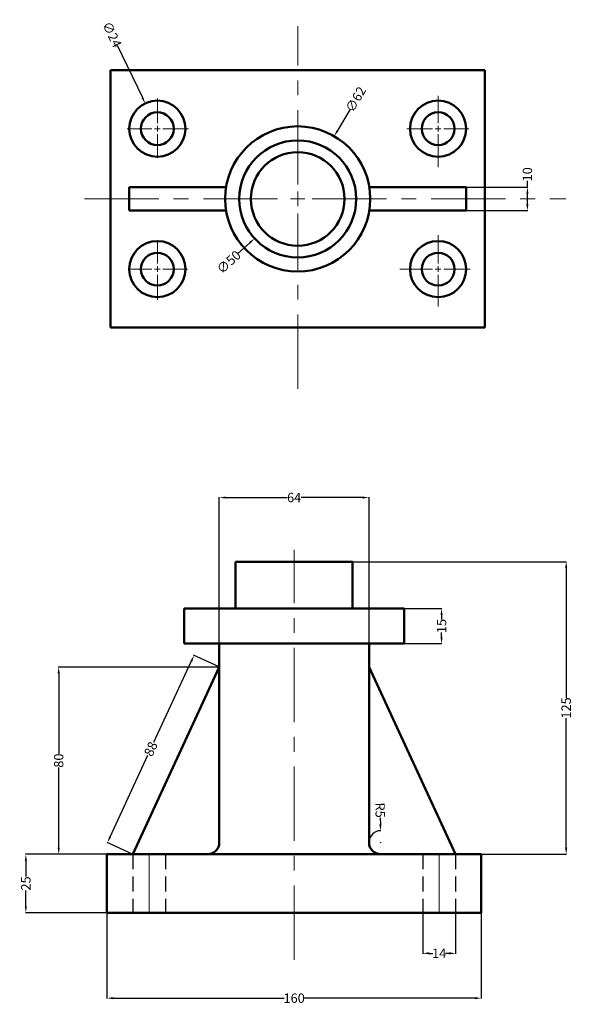
# Model space of a CAD drawing. Units: inches. Extents: x 680 to 916, y 368 to 789.
import ezdxf

# ---------------------------------------------------------------- set-up
doc = ezdxf.new("R2010")
doc.units = ezdxf.units.IN
doc.header["$MEASUREMENT"] = 0
doc.linetypes.add('CENTER', pattern=[50.8, 31.75, -6.35, 6.35, -6.35])
doc.linetypes.add('HIDDEN', pattern=[9.525, 6.35, -3.175])
for name, color, linetype, lineweight in [('M-CNTR', 1, 'CENTER', 18), ('M-DIMS', 2, 'Continuous', 25), ('M-HIDN', 6, 'HIDDEN', 25), ('M-OUTL', 7, 'Continuous', 50)]:
    doc.layers.add(name, color=color, linetype=linetype, lineweight=lineweight)
doc.styles.get("Standard").update_dxf_attribs({"font": 'arial.ttf'})
doc.dimstyles.get("Standard").update_dxf_attribs({"dimtxt": 4, "dimasz": 2.75, "dimexe": 0.18, "dimexo": 0.0625, "dimgap": 0.09, "dimtad": 0, "dimdec": 0, "dimzin": 0, "dimdsep": 46, "dimtxsty": 'Standard', "dimcen": 0.09, "dimadec": 0, "dimazin": 0, "dimtfac": 1, "dimtdec": 0, "dimtofl": 0, "dimtmove": 0, "dimatfit": 3, "dimfxl": 1, "dimtolj": 1, "dimtzin": 0, "dimarcsym": 0})

# ---------------------------------------------------------------- blocks, each defined once
blk = doc.blocks.new('*U1')
at = {"layer": 'M-CNTR', "color": 0, "transparency": 16777216}
for p, q in [((0, 2.4), (0, 12.94)), ((-12.91, 0), (-2.4, 0)), ((2.4, 0), (13.36, 0)), ((0, -12.46), (0, -2.4))]:
    blk.add_line(p, q, dxfattribs=at)
at = {"layer": 'M-CNTR', "color": 0, "linetype": 'Continuous', "transparency": 16777216}
for p, q in [((-1.2, 0), (1.2, 0)), ((0, -1.2), (0, 1.2))]:
    blk.add_line(p, q, dxfattribs=at)
blk = doc.blocks.new('*U2')
at = {"layer": 'M-CNTR', "color": 0, "transparency": 16777216}
for p, q in [((0, 2.4), (0, 12.35)), ((-12.5, 0), (-2.4, 0)), ((2.4, 0), (12.96, 0)), ((0, -13.15), (0, -2.4))]:
    blk.add_line(p, q, dxfattribs=at)
at = {"layer": 'M-CNTR', "color": 0, "linetype": 'Continuous', "transparency": 16777216}
for p, q in [((-1.2, 0), (1.2, 0)), ((0, -1.2), (0, 1.2))]:
    blk.add_line(p, q, dxfattribs=at)
blk = doc.blocks.new('*U3')
at = {"layer": 'M-CNTR', "color": 0, "transparency": 16777216}
for p, q in [((0, 2.4), (0, 14.5)), ((-16.29, 0), (-2.4, 0)), ((2.4, 0), (13.65, 0)), ((0, -15.95), (0, -2.4))]:
    blk.add_line(p, q, dxfattribs=at)
at = {"layer": 'M-CNTR', "color": 0, "linetype": 'Continuous', "transparency": 16777216}
for p, q in [((-1.2, 0), (1.2, 0)), ((0, -1.2), (0, 1.2))]:
    blk.add_line(p, q, dxfattribs=at)
blk = doc.blocks.new('*U4')
at = {"layer": 'M-CNTR', "color": 0, "transparency": 16777216}
for p, q in [((0, 2.4), (0, 13.99)), ((-13.32, 0), (-2.4, 0)), ((2.4, 0), (13.15, 0)), ((0, -16.48), (0, -2.4))]:
    blk.add_line(p, q, dxfattribs=at)
at = {"layer": 'M-CNTR', "color": 0, "linetype": 'Continuous', "transparency": 16777216}
for p, q in [((-1.2, 0), (1.2, 0)), ((0, -1.2), (0, 1.2))]:
    blk.add_line(p, q, dxfattribs=at)
blk = doc.blocks.new('*U5')
at = {"layer": 'M-CNTR', "color": 0, "transparency": 16777216}
for p, q in [((0, 6.2), (0, 73.87)), ((-91.14, 0), (-6.2, 0)), ((6.2, 0), (114.65, 0)), ((0, -81.14), (0, -6.2))]:
    blk.add_line(p, q, dxfattribs=at)
at = {"layer": 'M-CNTR', "color": 0, "linetype": 'Continuous', "transparency": 16777216}
for p, q in [((-3.1, 0), (3.1, 0)), ((0, -3.1), (0, 3.1))]:
    blk.add_line(p, q, dxfattribs=at)
blk = doc.blocks.new('*D6')
at = {"layer": 'Defpoints', "color": 0, "transparency": 16777216}
for p in [(871.07, 717.23), (897.24, 717.23), (871.07, 707.23)]:
    blk.add_point(p, dxfattribs=at)
at = {"layer": 'M-DIMS', "color": 0, "lineweight": -2, "transparency": 16777216}
for p, q in [((897.24, 717.23), (897.24, 719.98)), ((871.13, 717.23), (897.42, 717.23)), ((897.24, 709.98), (897.24, 714.48)), ((871.13, 707.23), (897.42, 707.23))]:
    blk.add_line(p, q, dxfattribs=at)
at = {"layer": 'M-DIMS', "color": 0, "transparency": 16777216}
for points in [[(896.78, 714.48), (897.7, 714.48), (897.24, 717.23)], [(896.78, 709.98), (897.7, 709.98), (897.24, 707.23)]]:
    blk.add_solid(points, dxfattribs=at)
at = {"layer": 'M-DIMS', "color": 0, "transparency": 16777216, "insert": (897.24, 722.74), "char_height": 4, "attachment_point": 5, "rotation": 90}
blk.add_mtext('\\A1;10', dxfattribs=at)
blk = doc.blocks.new('*D7')
at = {"layer": 'Defpoints', "color": 0, "transparency": 16777216}
for p in [(814.69, 739.04), (783.44, 685.43)]:
    blk.add_point(p, dxfattribs=at)
at = {"layer": 'M-DIMS', "color": 0, "lineweight": -2, "transparency": 16777216}
for p, q in [((821.28, 750.35), (816.07, 741.41)), ((798.98, 712.23), (799.16, 712.23)), ((799.07, 712.14), (799.07, 712.32))]:
    blk.add_line(p, q, dxfattribs=at)
at = {"layer": 'M-DIMS', "color": 0, "transparency": 16777216}
blk.add_solid([(815.68, 741.64), (816.47, 741.18), (814.69, 739.04)], dxfattribs=at)
at = {"layer": 'M-DIMS', "color": 0, "transparency": 16777216, "insert": (823.85, 754.76), "char_height": 4, "attachment_point": 5, "rotation": 59.7637}
blk.add_mtext('\\A1;∅62', dxfattribs=at)
blk = doc.blocks.new('*D8')
at = {"layer": 'Defpoints', "color": 0, "transparency": 16777216}
for p in [(817.5, 729.12), (780.63, 695.35)]:
    blk.add_point(p, dxfattribs=at)
at = {"layer": 'M-DIMS', "color": 0, "lineweight": -2, "transparency": 16777216}
for p, q in [((798.98, 712.23), (799.16, 712.23)), ((799.07, 712.14), (799.07, 712.32)), ((773.36, 688.7), (778.6, 693.49))]:
    blk.add_line(p, q, dxfattribs=at)
at = {"layer": 'M-DIMS', "color": 0, "transparency": 16777216}
blk.add_solid([(778.29, 693.83), (778.91, 693.15), (780.63, 695.35)], dxfattribs=at)
at = {"layer": 'M-DIMS', "color": 0, "transparency": 16777216, "insert": (769.58, 685.24), "char_height": 4, "attachment_point": 5, "rotation": 42.4796}
blk.add_mtext('\\A1;∅50', dxfattribs=at)
blk = doc.blocks.new('*D9')
at = {"layer": 'Defpoints', "color": 0, "transparency": 16777216}
for p in [(733.86, 753.05), (744.27, 731.42)]:
    blk.add_point(p, dxfattribs=at)
at = {"layer": 'M-DIMS', "color": 0, "lineweight": -2, "transparency": 16777216}
for p, q in [((721.91, 777.88), (732.67, 755.52)), ((738.98, 742.23), (739.16, 742.23)), ((739.07, 742.14), (739.07, 742.32))]:
    blk.add_line(p, q, dxfattribs=at)
at = {"layer": 'M-DIMS', "color": 0, "transparency": 16777216}
blk.add_solid([(733.08, 755.72), (732.26, 755.33), (733.86, 753.05)], dxfattribs=at)
at = {"layer": 'M-DIMS', "color": 0, "transparency": 16777216, "insert": (719.69, 782.49), "char_height": 4, "attachment_point": 5, "rotation": 295.7004}
blk.add_mtext('\\A1;∅24', dxfattribs=at)
blk = doc.blocks.new('*U10')
at = {"layer": 'M-CNTR', "color": 0, "transparency": 16777216}
blk.add_line((0, -87.62), (0, 87.62), dxfattribs=at)
blk = doc.blocks.new('*D11')
at = {"layer": 'Defpoints', "color": 0, "transparency": 16777216}
for p in [(829.54, 584.6), (765.54, 522.18), (829.54, 522.18)]:
    blk.add_point(p, dxfattribs=at)
at = {"layer": 'M-DIMS', "color": 0, "lineweight": -2, "transparency": 16777216}
for p, q in [((765.54, 522.24), (765.54, 584.78)), ((768.29, 584.6), (794.58, 584.6)), ((826.79, 584.6), (800.5, 584.6)), ((829.54, 522.24), (829.54, 584.78))]:
    blk.add_line(p, q, dxfattribs=at)
at = {"layer": 'M-DIMS', "color": 0, "transparency": 16777216}
for points in [[(768.29, 585.06), (768.29, 584.15), (765.54, 584.6)], [(826.79, 585.06), (826.79, 584.15), (829.54, 584.6)]]:
    blk.add_solid(points, dxfattribs=at)
at = {"layer": 'M-DIMS', "color": 0, "transparency": 16777216, "insert": (797.54, 584.6), "char_height": 4, "attachment_point": 5}
blk.add_mtext('\\A1;64', dxfattribs=at)
blk = doc.blocks.new('*D12')
at = {"layer": 'Defpoints', "color": 0, "transparency": 16777216}
for p in [(765.54, 512.18), (696.9, 432.18), (765.54, 432.18)]:
    blk.add_point(p, dxfattribs=at)
at = {"layer": 'M-DIMS', "color": 0, "lineweight": -2, "transparency": 16777216}
for p, q in [((765.48, 512.18), (696.72, 512.18)), ((696.9, 509.43), (696.9, 475.13)), ((696.9, 434.93), (696.9, 469.23)), ((765.48, 432.18), (696.72, 432.18))]:
    blk.add_line(p, q, dxfattribs=at)
at = {"layer": 'M-DIMS', "color": 0, "transparency": 16777216}
for points in [[(696.44, 509.43), (697.36, 509.43), (696.9, 512.18)], [(696.44, 434.93), (697.36, 434.93), (696.9, 432.18)]]:
    blk.add_solid(points, dxfattribs=at)
at = {"layer": 'M-DIMS', "color": 0, "transparency": 16777216, "insert": (696.9, 472.18), "char_height": 4, "attachment_point": 5, "rotation": 90}
blk.add_mtext('\\A1;80', dxfattribs=at)
blk = doc.blocks.new('*D13')
at = {"layer": 'Defpoints', "color": 0, "transparency": 16777216}
for p in [(765.54, 512.18), (717.75, 437.17), (728.54, 432.18)]:
    blk.add_point(p, dxfattribs=at)
at = {"layer": 'M-DIMS', "color": 0, "lineweight": -2, "transparency": 16777216}
for p, q in [((753.59, 514.67), (737.49, 479.85)), ((765.48, 512.2), (754.59, 517.24)), ((718.9, 439.66), (735.01, 474.48)), ((728.48, 432.2), (717.59, 437.24))]:
    blk.add_line(p, q, dxfattribs=at)
at = {"layer": 'M-DIMS', "color": 0, "transparency": 16777216}
for points in [[(753.18, 514.86), (754.01, 514.48), (754.75, 517.17)], [(718.49, 439.85), (719.32, 439.47), (717.75, 437.17)]]:
    blk.add_solid(points, dxfattribs=at)
at = {"layer": 'M-DIMS', "color": 0, "transparency": 16777216, "insert": (736.25, 477.17), "char_height": 4, "attachment_point": 5, "rotation": 65.1795}
blk.add_mtext('\\A1;88', dxfattribs=at)
blk = doc.blocks.new('*D14')
at = {"layer": 'Defpoints', "color": 0, "transparency": 16777216}
for p in [(717.54, 432.18), (682.86, 407.18), (717.54, 407.18)]:
    blk.add_point(p, dxfattribs=at)
at = {"layer": 'M-DIMS', "color": 0, "lineweight": -2, "transparency": 16777216}
for p, q in [((717.48, 432.18), (682.68, 432.18)), ((682.86, 429.43), (682.86, 422.68)), ((682.86, 409.93), (682.86, 416.67)), ((717.48, 407.18), (682.68, 407.18))]:
    blk.add_line(p, q, dxfattribs=at)
at = {"layer": 'M-DIMS', "color": 0, "transparency": 16777216}
for points in [[(682.4, 429.43), (683.32, 429.43), (682.86, 432.18)], [(682.4, 409.93), (683.32, 409.93), (682.86, 407.18)]]:
    blk.add_solid(points, dxfattribs=at)
at = {"layer": 'M-DIMS', "color": 0, "transparency": 16777216, "insert": (682.86, 419.68), "char_height": 4, "attachment_point": 5, "rotation": 90}
blk.add_mtext('\\A1;25', dxfattribs=at)
blk = doc.blocks.new('*D15')
at = {"layer": 'Defpoints', "color": 0, "transparency": 16777216}
for p in [(717.54, 407.18), (877.54, 407.18), (877.54, 370.65)]:
    blk.add_point(p, dxfattribs=at)
at = {"layer": 'M-DIMS', "color": 0, "lineweight": -2, "transparency": 16777216}
for p, q in [((717.54, 407.11), (717.54, 370.47)), ((877.54, 407.11), (877.54, 370.47)), ((720.29, 370.65), (793.22, 370.65)), ((874.79, 370.65), (801.85, 370.65))]:
    blk.add_line(p, q, dxfattribs=at)
at = {"layer": 'M-DIMS', "color": 0, "transparency": 16777216}
for points in [[(720.29, 371.11), (720.29, 370.19), (717.54, 370.65)], [(874.79, 371.11), (874.79, 370.19), (877.54, 370.65)]]:
    blk.add_solid(points, dxfattribs=at)
at = {"layer": 'M-DIMS', "color": 0, "transparency": 16777216, "insert": (797.54, 370.65), "char_height": 4, "attachment_point": 5}
blk.add_mtext('\\A1;160', dxfattribs=at)
blk = doc.blocks.new('*D16')
at = {"layer": 'Defpoints', "color": 0, "transparency": 16777216}
for p in [(852.54, 407.18), (866.54, 407.18), (866.54, 389.81)]:
    blk.add_point(p, dxfattribs=at)
at = {"layer": 'M-DIMS', "color": 0, "lineweight": -2, "transparency": 16777216}
for p, q in [((852.54, 407.11), (852.54, 389.63)), ((866.54, 407.11), (866.54, 389.63)), ((855.29, 389.81), (856.78, 389.81)), ((863.79, 389.81), (862.3, 389.81))]:
    blk.add_line(p, q, dxfattribs=at)
at = {"layer": 'M-DIMS', "color": 0, "transparency": 16777216}
for points in [[(855.29, 390.27), (855.29, 389.35), (852.54, 389.81)], [(863.79, 390.27), (863.79, 389.35), (866.54, 389.81)]]:
    blk.add_solid(points, dxfattribs=at)
at = {"layer": 'M-DIMS', "color": 0, "transparency": 16777216, "insert": (859.54, 389.81), "char_height": 4, "attachment_point": 5}
blk.add_mtext('\\A1;14', dxfattribs=at)
blk = doc.blocks.new('*D17')
at = {"layer": 'Defpoints', "color": 0, "transparency": 16777216}
for p in [(844.54, 537.18), (844.54, 522.18), (860.55, 522.18)]:
    blk.add_point(p, dxfattribs=at)
at = {"layer": 'M-DIMS', "color": 0, "lineweight": -2, "transparency": 16777216}
for p, q in [((844.6, 537.18), (860.73, 537.18)), ((860.55, 534.43), (860.55, 532.46)), ((860.55, 524.93), (860.55, 526.89)), ((844.6, 522.18), (860.73, 522.18))]:
    blk.add_line(p, q, dxfattribs=at)
at = {"layer": 'M-DIMS', "color": 0, "transparency": 16777216}
for points in [[(860.09, 534.43), (861.01, 534.43), (860.55, 537.18)], [(860.09, 524.93), (861.01, 524.93), (860.55, 522.18)]]:
    blk.add_solid(points, dxfattribs=at)
at = {"layer": 'M-DIMS', "color": 0, "transparency": 16777216, "insert": (860.55, 529.68), "char_height": 4, "attachment_point": 5, "rotation": 90}
blk.add_mtext('\\A1;15', dxfattribs=at)
blk = doc.blocks.new('*D18')
at = {"layer": 'Defpoints', "color": 0, "transparency": 16777216}
for p in [(834.46, 442.18), (834.54, 437.18)]:
    blk.add_point(p, dxfattribs=at)
at = {"layer": 'M-DIMS', "color": 0, "lineweight": -2, "transparency": 16777216}
for p, q in [((834.37, 447.68), (834.41, 444.93)), ((834.45, 437.18), (834.63, 437.18)), ((834.54, 437.09), (834.54, 437.27))]:
    blk.add_line(p, q, dxfattribs=at)
blk.add_arc((834.54, 437.18), 5, 88.8565, 179.2838, dxfattribs=at)
at = {"layer": 'M-DIMS', "color": 0, "transparency": 16777216}
blk.add_solid([(834.87, 444.93), (833.96, 444.92), (834.46, 442.18)], dxfattribs=at)
at = {"layer": 'M-DIMS', "color": 0, "transparency": 16777216, "insert": (834.32, 451), "char_height": 4, "attachment_point": 5, "rotation": 270.9191}
blk.add_mtext('\\A1;R5', dxfattribs=at)
blk = doc.blocks.new('*D19')
at = {"layer": 'Defpoints', "color": 0, "transparency": 16777216}
for p in [(797.54, 557.18), (797.54, 432.18), (913.81, 432.18)]:
    blk.add_point(p, dxfattribs=at)
at = {"layer": 'M-DIMS', "color": 0, "lineweight": -2, "transparency": 16777216}
for p, q in [((797.6, 557.18), (913.99, 557.18)), ((913.81, 554.43), (913.81, 499.01)), ((913.81, 434.93), (913.81, 490.34)), ((797.6, 432.18), (913.99, 432.18))]:
    blk.add_line(p, q, dxfattribs=at)
at = {"layer": 'M-DIMS', "color": 0, "transparency": 16777216}
for points in [[(913.35, 554.43), (914.27, 554.43), (913.81, 557.18)], [(913.35, 434.93), (914.27, 434.93), (913.81, 432.18)]]:
    blk.add_solid(points, dxfattribs=at)
at = {"layer": 'M-DIMS', "color": 0, "transparency": 16777216, "insert": (913.81, 494.68), "char_height": 4, "attachment_point": 5, "rotation": 90}
blk.add_mtext('\\A1;125', dxfattribs=at)
blk = doc.blocks.new('HOLE-CBORE')
for radius in [12, 7]:
    blk.add_circle((739.07, 682.23), radius)

msp = doc.modelspace()

# ---------------------------------------------------------------- linework, layer by layer
at = {"layer": 'M-CNTR'}
for p, q in [((735.54, 432.18), (735.54, 407.18)), ((859.54, 432.18), (859.54, 407.18))]:
    msp.add_line(p, q, dxfattribs=at)
at = {"layer": 'M-HIDN'}
for p, q in [((728.54, 432.18), (728.54, 407.18)), ((742.54, 432.18), (742.54, 407.18)), ((852.54, 432.18), (852.54, 407.18)), ((866.54, 432.18), (866.54, 407.18))]:
    msp.add_line(p, q, dxfattribs=at)
at = {"layer": 'M-OUTL'}
for p, q in [((879.07, 767.23), (719.07, 767.23)), ((719.07, 767.23), (719.07, 657.23)), ((879.07, 657.23), (879.07, 767.23)), ((727.07, 717.23), (727.07, 707.23)), ((768.45, 717.23), (727.07, 717.23)), ((871.07, 717.23), (829.68, 717.23)), ((871.07, 707.23), (871.07, 717.23)), ((768.45, 707.23), (727.07, 707.23)), ((871.07, 707.23), (829.68, 707.23)), ((719.07, 657.23), (879.07, 657.23)), ((799.07, 657.23), (739.07, 657.23)), ((772.54, 537.18), (772.54, 557.18)), ((772.54, 557.18), (822.54, 557.18)), ((822.54, 537.18), (822.54, 557.18)), ((750.54, 532.18), (750.54, 537.18)), ((750.54, 532.18), (750.54, 537.18)), ((750.54, 537.18), (822.54, 537.18)), ((844.54, 537.18), (822.54, 537.18)), ((844.54, 532.18), (844.54, 537.18)), ((750.54, 522.18), (750.54, 532.18)), ((750.54, 522.18), (750.54, 532.18)), ((844.54, 522.18), (844.54, 532.18)), ((829.54, 522.18), (750.54, 522.18)), ((829.54, 522.18), (750.54, 522.18)), ((765.54, 512.18), (765.54, 522.18)), ((829.54, 512.18), (829.54, 522.18)), ((829.54, 522.18), (844.54, 522.18)), ((765.54, 512.18), (728.54, 432.18)), ((765.54, 437.18), (765.54, 512.18)), ((829.54, 437.18), (829.54, 512.18)), ((866.54, 432.18), (829.54, 512.18)), ((717.54, 432.18), (717.54, 407.18)), ((717.54, 407.18), (717.54, 432.18)), ((717.54, 432.18), (834.54, 432.18)), ((717.54, 432.18), (742.54, 432.18)), ((877.54, 432.18), (834.54, 432.18)), ((877.54, 432.18), (852.54, 432.18)), ((877.54, 407.18), (877.54, 432.18)), ((717.54, 407.18), (877.54, 407.18))]:
    msp.add_line(p, q, dxfattribs=at)
for radius in [31.02, 25, 20]:
    msp.add_circle((799.07, 712.23), radius, dxfattribs=at)
for centre, start, end in [((760.54, 437.18), 270, 0), ((834.54, 437.18), 180, 270)]:
    msp.add_arc(centre, 5, start, end, dxfattribs=at)

# ---------------------------------------------------------------- block references
at = {"layer": 'M-CNTR'}
for name, p in [('*U5', (799.07, 712.23)), ('*U1', (739.07, 742.23)), ('*U4', (859.07, 742.23)), ('*U2', (739.07, 682.23)), ('*U3', (859.07, 682.23)), ('*U10', (797.54, 474.68))]:
    msp.add_blockref(name, p, dxfattribs=at)
at = {"layer": 'M-OUTL'}
for p in [(0, 60), (120, 60), (0, 0), (120, 0)]:
    msp.add_blockref('HOLE-CBORE', p, dxfattribs=at)

# ---------------------------------------------------------------- dimensions: what is measured, and where the dimension line sits
at = {"layer": 'M-DIMS'}
for p1, p2, picture, middle in [((744.27, 731.42), (733.86, 753.05), '*D9', (719.69, 782.49)), ((783.44, 685.43), (814.69, 739.04), '*D7', (823.85, 754.76)), ((817.5, 729.12), (780.63, 695.35), '*D8', (769.58, 685.24))]:
    dim = msp.add_diameter_dim_2p(p1=p1, p2=p2, dimstyle='Standard', override={"dimclrd": 0, "dimclre": 0, "dimclrt": 0}, dxfattribs=at)
    dim.commit()
    dim.dimension.update_dxf_attribs({"geometry": picture, "text_midpoint": middle, "dimtype": 163})
for base, p1, p2, picture, middle in [((897.24, 717.23), (871.07, 707.23), (871.07, 717.23), '*D6', (897.24, 722.74)), ((913.81, 432.18), (797.54, 557.18), (797.54, 432.18), '*D19', (913.81, 494.68)), ((860.55, 522.18), (844.54, 537.18), (844.54, 522.18), '*D17', (860.55, 529.68)), ((696.9, 432.18), (765.54, 512.18), (765.54, 432.18), '*D12', (696.9, 472.18)), ((682.86, 407.18), (717.54, 432.18), (717.54, 407.18), '*D14', (682.86, 419.68))]:
    dim = msp.add_linear_dim(base=base, p1=p1, p2=p2, angle=90, dimstyle='Standard', override={"dimclrd": 0, "dimclre": 0, "dimclrt": 0}, dxfattribs=at)
    dim.commit()
    dim.dimension.update_dxf_attribs({"geometry": picture, "text_midpoint": middle})
for base, p1, p2, picture, middle in [((829.54, 584.6), (765.54, 522.18), (829.54, 522.18), '*D11', (797.54, 584.6)), ((877.54, 370.65), (717.54, 407.18), (877.54, 407.18), '*D15', (797.54, 370.65)), ((866.54, 389.81), (852.54, 407.18), (866.54, 407.18), '*D16', (859.54, 389.81))]:
    dim = msp.add_linear_dim(base=base, p1=p1, p2=p2, dimstyle='Standard', override={"dimclrd": 0, "dimclre": 0, "dimclrt": 0}, dxfattribs=at)
    dim.commit()
    dim.dimension.update_dxf_attribs({"geometry": picture, "text_midpoint": middle})
dim = msp.add_aligned_dim(p1=(765.54, 512.18), p2=(728.54, 432.18), distance=-11.89, dimstyle='Standard', override={"dimclrd": 0, "dimclre": 0, "dimclrt": 0}, dxfattribs=at)
dim.commit()
dim.dimension.update_dxf_attribs({"geometry": '*D13', "text_midpoint": (736.25, 477.17)})
dim = msp.add_radius_dim(center=(834.54, 437.18), mpoint=(834.46, 442.18), dimstyle='Standard', override={"dimclrd": 0, "dimclre": 0, "dimclrt": 0}, dxfattribs=at)
dim.commit()
dim.dimension.update_dxf_attribs({"geometry": '*D18', "text_midpoint": (834.32, 451)})

doc.saveas('drawing.dxf')
